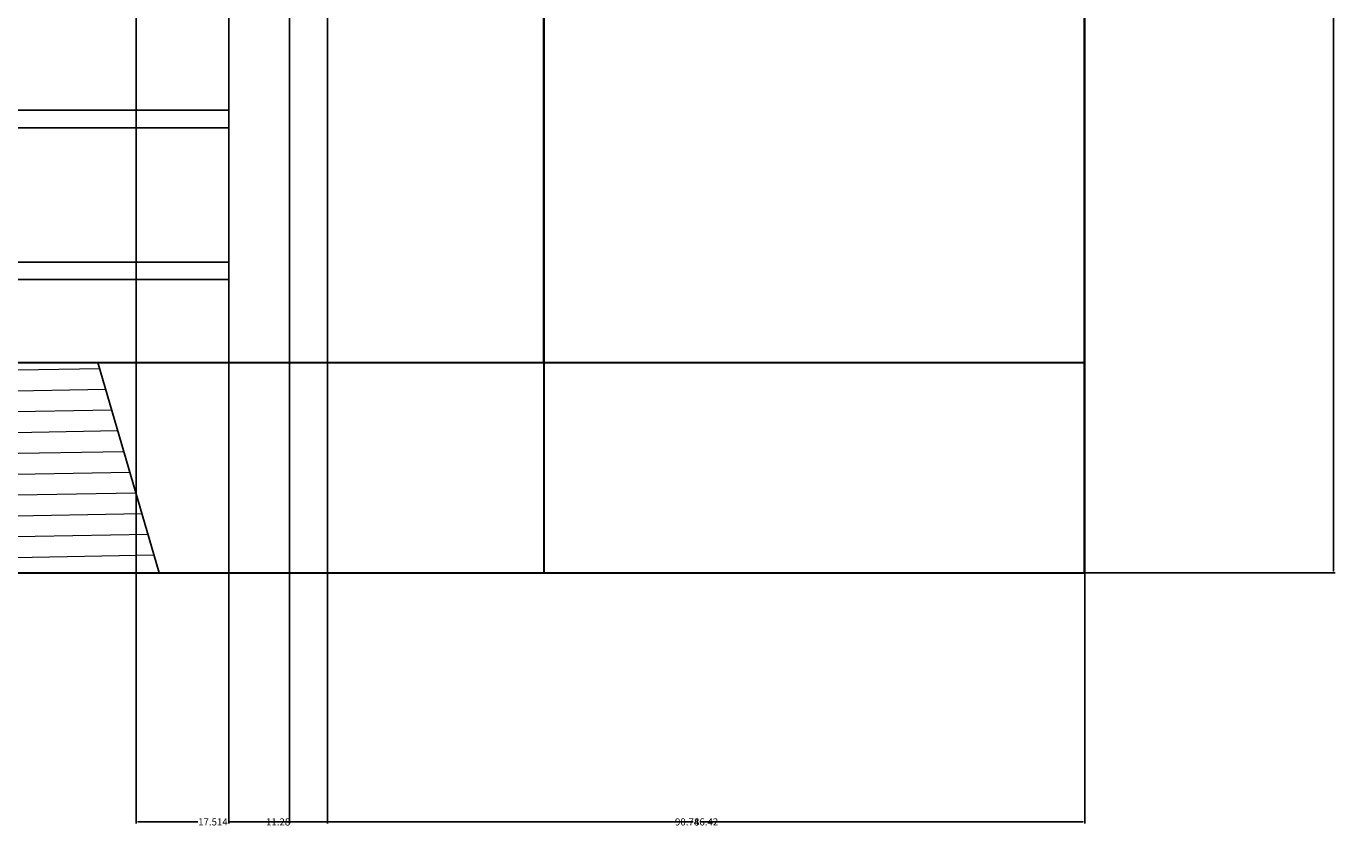
# Model space of a CAD drawing. Units: inches. Extents: x 69 to 650, y -16 to 573.
# Tile 9 of 26: x 499 to 649, y 35 to 126. Entities that reach past the tile are written whole.
import ezdxf

# ---------------------------------------------------------------- set-up
doc = ezdxf.new("R2010")
doc.units = ezdxf.units.IN
doc.header["$MEASUREMENT"] = 0
for name, color, linetype, lineweight in [('A-ANNO-DIMS', 2, 'Continuous', 18), ('A-COLS', 7, 'Continuous', 25), ('A-FLOR-PATT', 252, 'Continuous', 13), ('A-FLOR-STRS', 7, 'Continuous', 25), ('A-WALL', 7, 'Continuous', 35), ('A-WALL-BASE', 7, 'Continuous', 30)]:
    doc.layers.add(name, color=color, linetype=linetype, lineweight=lineweight)
doc.styles.get("Standard").update_dxf_attribs({"font": 'arial.ttf'})
doc.dimstyles.get("Standard").update_dxf_attribs({"dimtxt": 0.8125, "dimasz": 0.18, "dimexe": 0.18, "dimexo": 0.0625, "dimgap": 0.09, "dimtad": 0, "dimtih": 1, "dimtoh": 1, "dimdec": 4, "dimzin": 0, "dimdsep": 46, "dimlunit": 4, "dimtxsty": 'Standard', "dimcen": 0.09, "dimadec": 0, "dimazin": 0, "dimtfac": 1, "dimtdec": 4, "dimtofl": 0, "dimtmove": 0, "dimatfit": 3, "dimfxl": 1, "dimtolj": 1, "dimtzin": 0, "dimarcsym": 0})

# ---------------------------------------------------------------- blocks, each defined once
blk = doc.blocks.new('PIER-PORTAL-BANDED')
for p, q in [((0, 0), (0, 86.34)), ((0, 86.34), (26.94, 86.34)), ((0, 66.41), (26.94, 66.41)), ((0, 64.41), (26.94, 64.41)), ((0, 47.05), (26.94, 47.05)), ((0, 45.05), (26.94, 45.05)), ((0, 28.76), (26.94, 28.76)), ((0, 26.76), (26.94, 26.76)), ((0, 11.45), (26.94, 11.45)), ((0, 9.45), (26.94, 9.45))]:
    blk.add_line(p, q)
blk = doc.blocks.new('*D19')
at = {"layer": 'A-ANNO-DIMS', "color": 0, "lineweight": -2, "transparency": 16777216}
for p, q in [((99.56, 471.72), (99.56, 572.74)), ((99.74, 572.56), (358.57, 572.56)), ((619.38, 572.56), (360.54, 572.56)), ((619.56, 87.99), (619.56, 572.74))]:
    blk.add_line(p, q, dxfattribs=at)
at = {"layer": 'A-ANNO-DIMS', "color": 0, "transparency": 16777216}
for points in [[(99.74, 572.59), (99.74, 572.53), (99.56, 572.56)], [(619.38, 572.59), (619.38, 572.53), (619.56, 572.56)]]:
    blk.add_solid(points, dxfattribs=at)
at = {"layer": 'Defpoints', "color": 0, "transparency": 16777216}
for p in [(619.56, 572.56), (99.56, 471.66), (619.56, 87.93)]:
    blk.add_point(p, dxfattribs=at)
at = {"layer": 'A-ANNO-DIMS', "color": 0, "transparency": 16777216, "insert": (359.56, 572.56), "char_height": 0.812, "attachment_point": 5}
blk.add_mtext('\\A1;520', dxfattribs=at)
blk = doc.blocks.new('*D20')
at = {"layer": 'A-ANNO-DIMS', "color": 0, "lineweight": -2, "transparency": 16777216}
for p, q in [((504.24, 544.16), (648.14, 544.16)), ((647.96, 543.98), (647.96, 304.55)), ((647.96, 64.11), (647.96, 303.54)), ((619.62, 63.93), (648.14, 63.93))]:
    blk.add_line(p, q, dxfattribs=at)
at = {"layer": 'A-ANNO-DIMS', "color": 0, "transparency": 16777216}
for points in [[(647.93, 543.98), (647.99, 543.98), (647.96, 544.16)], [(647.93, 64.11), (647.99, 64.11), (647.96, 63.93)]]:
    blk.add_solid(points, dxfattribs=at)
at = {"layer": 'Defpoints', "color": 0, "transparency": 16777216}
for p in [(504.18, 544.16), (647.96, 544.16), (619.56, 63.93)]:
    blk.add_point(p, dxfattribs=at)
at = {"layer": 'A-ANNO-DIMS', "color": 0, "transparency": 16777216, "insert": (647.96, 304.04), "char_height": 0.812, "attachment_point": 5}
blk.add_mtext('\\A1;480.2', dxfattribs=at)
blk = doc.blocks.new('*D33')
at = {"layer": 'A-ANNO-DIMS', "color": 0, "lineweight": -2, "transparency": 16777216}
for p, q in [((533.14, 174.2), (533.14, 35.35)), ((521.86, 87.87), (521.86, 35.35)), ((522.04, 35.53), (526.07, 35.53)), ((532.96, 35.53), (528.92, 35.53))]:
    blk.add_line(p, q, dxfattribs=at)
at = {"layer": 'A-ANNO-DIMS', "color": 0, "transparency": 16777216}
for points in [[(522.04, 35.56), (522.04, 35.5), (521.86, 35.53)], [(532.96, 35.56), (532.96, 35.5), (533.14, 35.53)]]:
    blk.add_solid(points, dxfattribs=at)
at = {"layer": 'Defpoints', "color": 0, "transparency": 16777216}
for p in [(533.14, 174.27), (521.86, 87.93), (533.14, 35.53)]:
    blk.add_point(p, dxfattribs=at)
at = {"layer": 'A-ANNO-DIMS', "color": 0, "transparency": 16777216, "insert": (527.5, 35.53), "char_height": 0.812, "attachment_point": 5}
blk.add_mtext('\\A1;11.28', dxfattribs=at)
blk = doc.blocks.new('*D34')
at = {"layer": 'A-ANNO-DIMS', "color": 0, "lineweight": -2, "transparency": 16777216}
for p, q in [((533.14, 174.2), (533.14, 35.35)), ((619.56, 87.87), (619.56, 35.35)), ((533.32, 35.53), (574.89, 35.53)), ((619.38, 35.53), (577.8, 35.53))]:
    blk.add_line(p, q, dxfattribs=at)
at = {"layer": 'A-ANNO-DIMS', "color": 0, "transparency": 16777216}
for points in [[(533.32, 35.56), (533.32, 35.5), (533.14, 35.53)], [(619.38, 35.56), (619.38, 35.5), (619.56, 35.53)]]:
    blk.add_solid(points, dxfattribs=at)
at = {"layer": 'Defpoints', "color": 0, "transparency": 16777216}
for p in [(533.14, 174.27), (619.56, 87.93), (619.56, 35.53)]:
    blk.add_point(p, dxfattribs=at)
at = {"layer": 'A-ANNO-DIMS', "color": 0, "transparency": 16777216, "insert": (576.35, 35.53), "char_height": 0.812, "attachment_point": 5}
blk.add_mtext('\\A1;86.42', dxfattribs=at)
blk = doc.blocks.new('*D40')
at = {"layer": 'A-ANNO-DIMS', "color": 0, "lineweight": -2, "transparency": 16777216}
for p, q in [((511.3, 372.93), (511.3, 35.35)), ((528.81, 243.87), (528.81, 35.35)), ((511.48, 35.53), (518.32, 35.53)), ((528.63, 35.53), (521.79, 35.53))]:
    blk.add_line(p, q, dxfattribs=at)
at = {"layer": 'A-ANNO-DIMS', "color": 0, "transparency": 16777216}
for points in [[(511.48, 35.56), (511.48, 35.5), (511.3, 35.53)], [(528.63, 35.56), (528.63, 35.5), (528.81, 35.53)]]:
    blk.add_solid(points, dxfattribs=at)
at = {"layer": 'Defpoints', "color": 0, "transparency": 16777216}
for p in [(511.3, 372.99), (528.81, 243.93), (528.81, 35.53)]:
    blk.add_point(p, dxfattribs=at)
at = {"layer": 'A-ANNO-DIMS', "color": 0, "transparency": 16777216, "insert": (520.06, 35.53), "char_height": 0.812, "attachment_point": 5}
blk.add_mtext('\\A1;17.514', dxfattribs=at)
blk = doc.blocks.new('*D41')
at = {"layer": 'A-ANNO-DIMS', "color": 0, "lineweight": -2, "transparency": 16777216}
for p, q in [((528.81, 243.87), (528.81, 35.35)), ((619.56, 243.87), (619.56, 35.35)), ((528.99, 35.53), (572.72, 35.53)), ((619.38, 35.53), (575.64, 35.53))]:
    blk.add_line(p, q, dxfattribs=at)
at = {"layer": 'A-ANNO-DIMS', "color": 0, "transparency": 16777216}
for points in [[(528.99, 35.56), (528.99, 35.5), (528.81, 35.53)], [(619.38, 35.56), (619.38, 35.5), (619.56, 35.53)]]:
    blk.add_solid(points, dxfattribs=at)
at = {"layer": 'Defpoints', "color": 0, "transparency": 16777216}
for p in [(528.81, 243.93), (619.56, 243.93), (619.56, 35.53)]:
    blk.add_point(p, dxfattribs=at)
at = {"layer": 'A-ANNO-DIMS', "color": 0, "transparency": 16777216, "insert": (574.18, 35.53), "char_height": 0.812, "attachment_point": 5}
blk.add_mtext('\\A1;90.74', dxfattribs=at)

msp = doc.modelspace()

# ---------------------------------------------------------------- hatches: boundary and pattern name
at = {"layer": 'A-FLOR-PATT'}
h = msp.add_hatch(dxfattribs=at)
h.set_pattern_fill('ANSI31', color=256, scale=19, angle=136)
h.paths.add_polyline_path([(506.932, 87.93), (463.7847, 87.93), (388.9646, 87.93), (372.9372, 87.93), (369.3072, 63.93), (463.7847, 63.93), (513.9402, 63.93)])

# ---------------------------------------------------------------- linework, layer by layer
at = {"layer": 'A-FLOR-STRS'}
msp.add_lwpolyline([(506.932, 87.93), (513.9402, 63.93)], dxfattribs=at)
at = {"layer": 'A-WALL'}
for p, q in [((619.555, 411.93), (619.555, 69.3788)), ((557.8179, 243.93), (557.8179, 87.93))]:
    msp.add_line(p, q, dxfattribs=at)
at = {"layer": 'A-WALL-BASE'}
for p, q in [((463.7847, 87.93), (557.8179, 87.93)), ((557.8179, 87.93), (557.8179, 63.93)), ((557.8179, 87.93), (619.555, 87.93)), ((619.555, 63.93), (619.555, 69.3788)), ((463.7847, 63.93), (557.8179, 63.93)), ((557.8179, 63.93), (619.555, 63.93))]:
    msp.add_line(p, q, dxfattribs=at)

# ---------------------------------------------------------------- block references
at = {"layer": 'A-COLS', "extrusion": (0, 0, -1), "zscale": -1}
msp.add_blockref('PIER-PORTAL-BANDED', (-521.8566, 87.93), dxfattribs=at)

# ---------------------------------------------------------------- dimensions: what is measured, and where the dimension line sits
at = {"layer": 'A-ANNO-DIMS'}
for base, p1, p2, override, picture, middle in [((619.555, 572.5573), (99.556, 471.6595), (619.555, 87.93), {"dimdec": 0, "dimlfac": 1, "dimrnd": 0, "dimzin": 0, "dimdsep": 46, "dimlunit": 2}, '*D19', (359.5555, 572.5573)), ((528.812, 35.53), (511.2984, 372.9907), (528.812, 243.93), {"dimdec": 3, "dimlfac": 1, "dimrnd": 0, "dimzin": 0, "dimdsep": 46, "dimlunit": 2}, '*D40', (520.0552, 35.53)), ((619.555, 35.53), (528.812, 243.93), (619.555, 243.93), {"dimdec": 2, "dimlfac": 1, "dimrnd": 0, "dimzin": 0, "dimdsep": 46, "dimlunit": 2}, '*D41', (574.1835, 35.53)), ((533.1369, 35.53), (521.8566, 87.93), (533.1369, 174.2666), {"dimdec": 2, "dimlfac": 1, "dimrnd": 0, "dimzin": 0, "dimdsep": 46, "dimlunit": 2}, '*D33', (527.4967, 35.53)), ((619.555, 35.53), (533.1369, 174.2666), (619.555, 87.93), {"dimdec": 2, "dimlfac": 1, "dimrnd": 0, "dimzin": 0, "dimdsep": 46, "dimlunit": 2}, '*D34', (576.3459, 35.53))]:
    dim = msp.add_linear_dim(base=base, p1=p1, p2=p2, dimstyle='Standard', override=override, dxfattribs=at)
    dim.commit()
    dim.dimension.update_dxf_attribs({"geometry": picture, "text_midpoint": middle})
dim = msp.add_linear_dim(base=(647.955, 544.1573), p1=(619.555, 63.93), p2=(504.1763, 544.1573), angle=90, dimstyle='Standard', override={"dimdec": 1, "dimlfac": 1, "dimrnd": 0, "dimzin": 0, "dimdsep": 46, "dimlunit": 2}, dxfattribs=at)
dim.commit()
dim.dimension.update_dxf_attribs({"geometry": '*D20', "text_midpoint": (647.955, 304.0436)})

doc.saveas('drawing.dxf')
